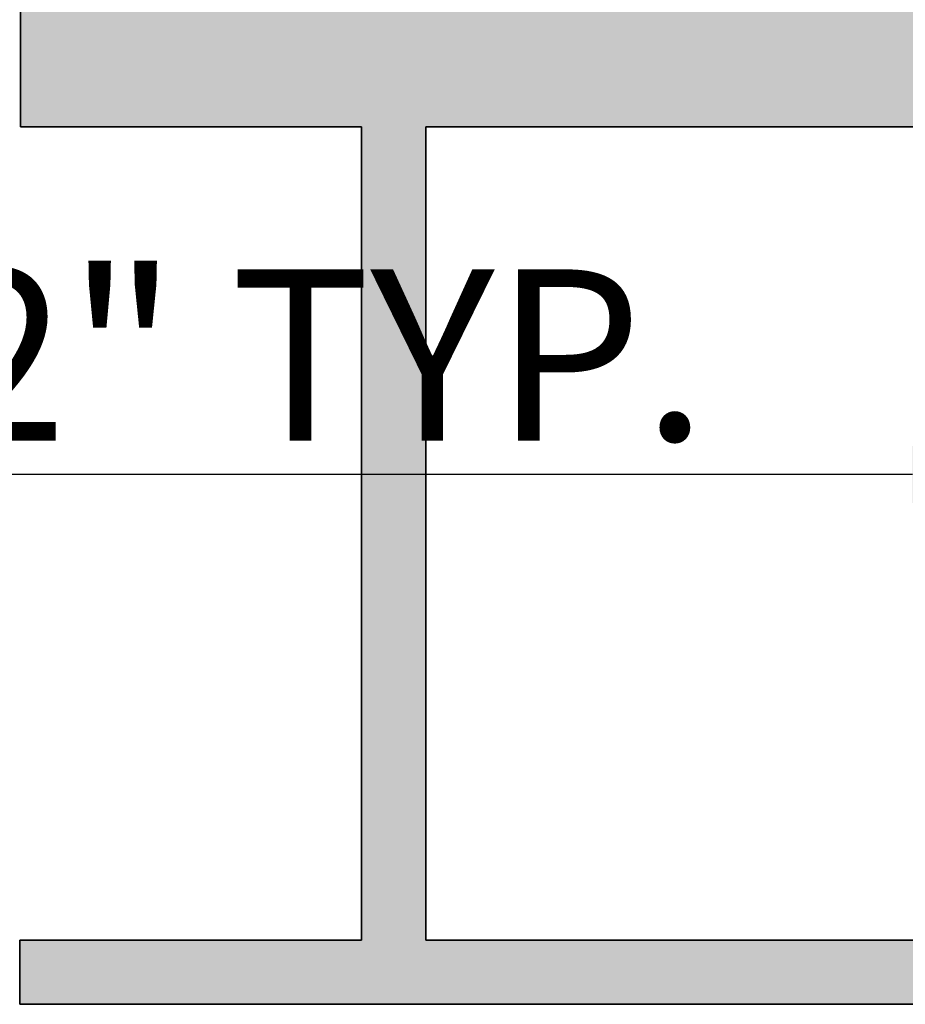
# Model space of a CAD drawing. Units: inches. Extents: x 2083 to 3317, y 1141 to 2115.
# Tile 246 of 256: x 2944 to 3006, y 1416 to 1485. Entities that reach past the tile are written whole.
import ezdxf

# ---------------------------------------------------------------- set-up
doc = ezdxf.new("R2010")
doc.units = ezdxf.units.IN
doc.layers.add('A-ANNO-DIMS', color=2, linetype='Continuous', lineweight=18)
doc.layers.add('A-WALL', color=7, linetype='Continuous', lineweight=35)
doc.layers.add('A-WALL-PATT', color=251, linetype='Continuous', lineweight=13, true_color=0x636466)
doc.styles.get("Standard").update_dxf_attribs({"font": 'arial.ttf'})
doc.dimstyles.new('ISO-25', dxfattribs={"dimtxt": 12, "dimasz": 12, "dimexe": 1.25, "dimexo": 0.625, "dimtad": 1, "dimlunit": 3, "dimtxsty": 'Standard', "dimcen": 2.5, "dimadec": 0, "dimazin": 0, "dimtfac": 1, "dimtmove": 0, "dimatfit": 3, "dimfxl": 1, "dimarcsym": 0})

# ---------------------------------------------------------------- blocks, each defined once
blk = doc.blocks.new('*D18')
at = {"layer": 'A-ANNO-DIMS', "color": 0, "lineweight": -2, "transparency": 16777216}
for p, q in [((3018.476, 1456.156), (3018.476, 1452.142)), ((3041.068, 1456.156), (3041.068, 1452.142)), ((3006.476, 1453.392), (2828.361, 1453.392)), ((3041.068, 1453.392), (3018.476, 1453.392)), ((3053.068, 1453.392), (3065.068, 1453.392))]:
    blk.add_line(p, q, dxfattribs=at)
at = {"layer": 'A-ANNO-DIMS', "color": 0, "transparency": 16777216}
for points in [[(3006.476, 1455.392), (3006.476, 1451.392), (3018.476, 1453.392)], [(3053.068, 1455.392), (3053.068, 1451.392), (3041.068, 1453.392)]]:
    blk.add_solid(points, dxfattribs=at)
at = {"layer": 'Defpoints', "color": 0, "transparency": 16777216}
for p in [(3018.476, 1456.781), (3041.068, 1456.781), (3018.476, 1453.392)]:
    blk.add_point(p, dxfattribs=at)
at = {"layer": 'A-ANNO-DIMS', "color": 0, "transparency": 16777216, "insert": (2911.418, 1460.222), "char_height": 12, "attachment_point": 5}
blk.add_mtext('BASIN 1\'-10 1/2" TYP.', dxfattribs=at)
blk = doc.blocks.new('*D73')
at = {"layer": 'A-ANNO-DIMS', "color": 0, "lineweight": -2, "transparency": 16777216}
for p, q in [((2895.865, 1420.763), (2930.553, 1387.52)), ((2980.105, 1340.032), (2939.217, 1379.217))]:
    blk.add_line(p, q, dxfattribs=at)
at = {"layer": 'A-ANNO-DIMS', "color": 0, "transparency": 16777216}
blk.add_solid([(2940.601, 1380.661), (2937.833, 1377.773), (2930.553, 1387.52)], dxfattribs=at)
at = {"layer": 'Defpoints', "color": 0, "transparency": 16777216}
for p in [(2895.865, 1420.763), (2930.553, 1387.52)]:
    blk.add_point(p, dxfattribs=at)
at = {"layer": 'A-ANNO-DIMS', "color": 0, "transparency": 16777216, "insert": (2968.665, 1360.348), "char_height": 12, "attachment_point": 5, "rotation": 316.21871}
blk.add_mtext('R4\'-0"', dxfattribs=at)

msp = doc.modelspace()

# ---------------------------------------------------------------- hatches: boundary and pattern name
at = {"layer": 'A-WALL-PATT'}
h = msp.add_hatch(color=256, dxfattribs=at)
h.dxf.hatch_style = 1
h.paths.add_polyline_path([(3126.96, 2020.761), (2748.96, 2020.761), (2604.96, 2020.761), (2226.96, 2020.761), (2226.96, 1702.761), (2466.96, 1702.761), (2466.96, 1582.761), (2418.96, 1582.761), (2418.96, 1477.761), (2226.96, 1477.761), (2226.96, 1263.261), (2544.96, 1263.261), (2544.96, 1411.761), (2604.96, 1411.761), (2685.96, 1411.761), (2685.96, 1420.761), (2604.96, 1420.761), (2604.96, 1573.761), (2604.96, 1702.761), (2604.96, 2011.761), (2748.96, 2011.761), (2748.96, 1702.761), (2862.96, 1702.761), (2862.96, 1621.761), (2871.96, 1621.761), (2871.96, 1702.761), (2883.96, 1702.761), (2883.96, 1706.939, -0.026459), (2883.96, 1711.761), (2757.96, 1711.761), (2757.96, 1807.761), (2787.96, 1807.761), (2787.96, 1812.261), (2757.96, 1812.261), (2757.96, 2011.761), (2877.96, 2011.761), (2877.96, 1812.261), (2847.96, 1812.261), (2847.96, 1807.761), (2889.836, 1807.761), (2889.836, 1812.261), (2882.46, 1812.261), (2882.46, 2011.761), (3117.96, 2011.761), (3117.96, 1812.261), (2937.836, 1812.261), (2937.836, 1807.761), (2995.71, 1807.761), (2995.71, 1796.118), (3000.21, 1796.118), (3000.21, 1807.761), (3117.96, 1807.761), (3117.96, 1711.761), (3000.21, 1711.761), (3000.21, 1760.118), (2998.573, 1760.118, -0.020711), (2995.71, 1760.118), (2995.71, 1711.761), (2931.96, 1711.761), (2931.96, 1702.761), (3126.96, 1702.761)])
h.paths.add_polyline_path([(2471.46, 2011.761), (2471.46, 1810.011), (2462.717, 1810.011), (2462.717, 1805.511), (2505.96, 1805.511), (2505.96, 1810.011), (2475.96, 1810.011), (2475.96, 2011.761), (2595.96, 2011.761), (2595.96, 1810.011), (2565.96, 1810.011), (2565.96, 1805.511), (2595.96, 1805.511), (2595.96, 1711.761), (2235.96, 1711.761), (2235.96, 1805.511), (2353.71, 1805.511), (2353.71, 1796.054), (2358.21, 1796.054), (2358.21, 1805.511), (2414.717, 1805.511), (2414.717, 1810.011), (2235.96, 1810.011), (2235.96, 2011.761)], flags=16)
h.paths.add_polyline_path([(2270.205, 1994.61), (2270.205, 1970.61), (2246.205, 1970.61), (2246.205, 1994.61)], flags=0)
edge = h.paths.add_edge_path(flags=0)
edge.add_ellipse((2332.027, 1899.798), major_axis=(-3.043, 3.043), ratio=0.168252, start_angle=-161.33217, end_angle=-156.30711, ccw=False)
edge.add_ellipse((2333.082, 1898.744), major_axis=(-1.055, 1.055), ratio=0.453532, start_angle=-123.37102, end_angle=-94.15911)
edge = h.paths.add_edge_path(flags=0)
edge.add_ellipse((2332.027, 1968.876), major_axis=(3.043, 3.043), ratio=0.168252, start_angle=18.66783, end_angle=23.69289)
edge.add_spline(control_points=[(2332.926, 1970.691), (2332.227, 1970.336), (2330.894, 1969.659), (2328.413, 1970.932), (2327.204, 1967.749), (2324.71, 1969.956), (2322.533, 1967.012), (2320.013, 1971.296), (2317.68, 1968.158), (2316.041, 1967.102), (2315.427, 1966.81)], knot_values=[0, 0, 0, 0, 2.267059, 4.324559, 6.685584, 8.878641, 11.121502, 14.300359, 17.755284, 19.732645, 19.732645, 19.732645, 19.732645], degree=3, periodic=0)
edge.add_ellipse((2332.027, 1968.876), major_axis=(3.043, 3.043), ratio=0.168252, start_angle=18.66783, end_angle=23.69289, ccw=False)
edge.add_ellipse((2333.082, 1969.931), major_axis=(1.055, 1.055), ratio=0.453532, start_angle=56.62898, end_angle=85.84089, ccw=False)
edge = h.paths.add_edge_path(flags=0)
edge.add_spline(control_points=[(2296.428, 1967.988), (2293.628, 1965.336), (2287.704, 1959.727), (2299.744, 1949.996), (2294.533, 1935.669), (2290.573, 1920.604), (2293.394, 1909.974), (2296.185, 1904.967)], knot_values=[0.099185, 0.099185, 0.099185, 0.099185, 0.345301, 0.619822, 0.982653, 1.386093, 1.810555, 1.810555, 1.810555, 1.810555], degree=3, periodic=0)
edge.add_spline(control_points=[(2296.185, 1904.967), (2297.384, 1902.619), (2298.001, 1901.949), (2298.553, 1901.468)], knot_values=[0.006246, 0.006246, 0.006246, 0.006246, 0.055476, 0.055476, 0.055476, 0.055476], degree=3, periodic=0)
edge.add_spline(control_points=[(2298.553, 1901.468), (2297.259, 1900.923), (2295.225, 1900.232), (2293.06, 1900.614), (2292.101, 1900.788), (2292.09, 1900.791)], knot_values=[0.312835, 0.312835, 0.312835, 0.312835, 0.40178, 0.474987, 0.475903, 0.475903, 0.475903, 0.475903], degree=3, periodic=0)
edge.add_arc((2292.794, 1904.664), 3.937, 215.4209, 259.69818, ccw=False)
edge.add_spline(control_points=[(2289.585, 1902.382), (2289.477, 1902.535), (2289.368, 1902.688), (2289.261, 1902.841)], knot_values=[0.102872, 0.102872, 0.102872, 0.102872, 0.116896, 0.116896, 0.116896, 0.116896], degree=3, periodic=0)
edge.add_spline(control_points=[(2289.261, 1902.841), (2288.687, 1902.55), (2287.64, 1902.02), (2285.881, 1901.874), (2283.853, 1901.504), (2281.72, 1899.711), (2278.467, 1899.493), (2276.157, 1901.883), (2272.259, 1899.804), (2267.778, 1901.843), (2262.244, 1900.184), (2257.415, 1901.782), (2254.318, 1900.726), (2253.178, 1900.337)], knot_values=[0, 0, 0, 0, 1.907977, 3.477176, 5.261074, 7.972851, 11.680248, 13.717921, 16.939592, 22.789562, 27.502503, 33.595215, 37.145618, 37.145618, 37.145618, 37.145618], degree=3, periodic=0)
edge.add_line((2253.178, 1900.337), (2250.244, 1902.841))
edge.add_line((2250.244, 1902.841), (2250.244, 1965.833))
edge.add_line((2250.244, 1965.833), (2253.178, 1968.337))
edge.add_spline(control_points=[(2253.178, 1968.337), (2254.318, 1967.948), (2257.415, 1966.892), (2262.244, 1968.49), (2267.778, 1966.831), (2271.527, 1968.537), (2273.876, 1967.828), (2274.207, 1967.728)], knot_values=[0, 0, 0, 0, 0.09018, 0.244935, 0.364644, 0.513233, 0.537855, 0.537855, 0.537855, 0.537855], degree=3, periodic=0)
edge.add_arc((2274.353, 1963.793), 3.937, 72.05113, 92.12795, ccw=False)
edge.add_arc((2281.297, 1985.23), 18.596, 252.05113, 288.56572)
edge.add_arc((2292.317, 1956.029), 12.646, 71.02679, 113.77822, ccw=False)
edge = h.paths.add_edge_path(flags=0)
edge.add_spline(control_points=[(2274.899, 1951.856), (2275.066, 1951.617), (2275.233, 1951.377), (2275.398, 1951.136)], knot_values=[1.409916, 1.409916, 1.409916, 1.409916, 1.43159, 1.43159, 1.43159, 1.43159], degree=3, periodic=0)
edge.add_spline(control_points=[(2275.398, 1951.136), (2275.792, 1950.562), (2276.179, 1949.984), (2276.546, 1949.397)], knot_values=[1.358238, 1.358238, 1.358238, 1.358238, 1.409916, 1.409916, 1.409916, 1.409916], degree=3, periodic=0)
edge.add_line((2276.546, 1949.397), (2277.437, 1947.862))
edge.add_spline(control_points=[(2277.437, 1947.862), (2276.304, 1945.673), (2274.64, 1942.427), (2274.632, 1938.094), (2272.799, 1930.852), (2274.356, 1943.897), (2275.948, 1947.923), (2276.546, 1949.397)], knot_values=[0.005632, 0.005632, 0.005632, 0.005632, 0.186014, 0.266002, 0.357087, 0.59639, 0.739732, 0.739732, 0.739732, 0.739732], degree=3, periodic=0)
edge.add_spline(control_points=[(2276.546, 1949.397), (2276.179, 1949.984), (2275.792, 1950.562), (2275.398, 1951.136)], knot_values=[1.358238, 1.358238, 1.358238, 1.358238, 1.409916, 1.409916, 1.409916, 1.409916], degree=3, periodic=0)
edge.add_spline(control_points=[(2275.398, 1951.136), (2274.943, 1950.08), (2274.208, 1948.025), (2273.935, 1944.851), (2272.469, 1937.627), (2273.466, 1945.696), (2274.701, 1951.059), (2274.899, 1951.856)], knot_values=[0.104364, 0.104364, 0.104364, 0.104364, 0.189636, 0.269624, 0.36071, 0.600013, 0.644622, 0.644622, 0.644622, 0.644622], degree=3, periodic=0)
h.paths.add_polyline_path([(2269.168, 1963.128, -0.357527), (2268.171, 1960.976, -0.092561), (2268.171, 1939.436, -0.357527), (2269.168, 1937.285, -0.357527), (2267.016, 1938.282, -0.164785), (2254.686, 1938.282, -0.357527), (2252.534, 1937.285, -0.357527), (2253.531, 1939.436, -0.092561), (2253.531, 1960.976, -0.357527), (2252.534, 1963.128, -0.357527), (2254.686, 1962.131, -0.164785), (2267.016, 1962.131, -0.357527)], flags=0)
h.paths.add_polyline_path([(2248.874, 1967.802), (2248.874, 1957.028), (2249.458, 1957.028), (2249.458, 1911.647), (2248.874, 1911.647), (2248.874, 1900.873), (2246.512, 1900.873, 0.197327), (2244.15, 1902.457), (2244.15, 1966.218, 0.197327), (2246.512, 1967.802)], flags=0)
h.paths.add_polyline_path([(2269.168, 1931.389, -0.357527), (2268.171, 1929.238, -0.092561), (2268.171, 1907.698, -0.357527), (2269.168, 1905.547, -0.357527), (2267.016, 1906.544, -0.164785), (2254.686, 1906.544, -0.357527), (2252.534, 1905.547, -0.357527), (2253.531, 1907.698, -0.092561), (2253.531, 1929.238, -0.357527), (2252.534, 1931.389, -0.357527), (2254.686, 1930.392, -0.164785), (2267.016, 1930.392, -0.357527)], flags=0)
edge = h.paths.add_edge_path(flags=0)
edge.add_spline(control_points=[(2276.197, 1906.724), (2276.168, 1909.029), (2276.114, 1913.372), (2270.598, 1924.925), (2273.905, 1919.013), (2275.922, 1916.262), (2275.475, 1912.402), (2277.258, 1910.381), (2276.696, 1908.225), (2276.646, 1906.813), (2276.618, 1906.008)], knot_values=[0, 0, 0, 0, 8.61026, 16.221274, 18.843057, 23.804898, 27.440828, 29.356102, 31.203478, 33.650687, 33.650687, 33.650687, 33.650687], degree=3, periodic=0)
edge.add_spline(control_points=[(2276.618, 1906.008), (2276.623, 1905.624), (2276.498, 1904.629), (2275.442, 1903.855), (2274.937, 1903.08), (2274.859, 1902.841)], knot_values=[0.156488, 0.156488, 0.156488, 0.156488, 0.184398, 0.231376, 0.250598, 0.250598, 0.250598, 0.250598], degree=3, periodic=0)
edge.add_line((2274.859, 1902.841), (2276.506, 1902.841))
edge.add_spline(control_points=[(2276.506, 1902.841), (2276.788, 1903.085), (2277.665, 1904.125), (2278.25, 1904.341), (2277.654, 1908.527), (2278.156, 1906.228), (2278.1, 1905.286), (2278.847, 1904.069), (2277.857, 1903.415), (2277.874, 1902.991), (2277.904, 1902.841)], knot_values=[0.059574, 0.059574, 0.059574, 0.059574, 0.080753, 0.103741, 0.16972, 0.176036, 0.207137, 0.240474, 0.262341, 0.27366, 0.27366, 0.27366, 0.27366], degree=3, periodic=0)
edge.add_line((2277.904, 1902.841), (2280.03, 1902.841))
edge.add_spline(control_points=[(2280.03, 1902.841), (2279.888, 1903.088), (2279.499, 1903.982), (2280.152, 1905.939), (2278.104, 1909.658), (2279.762, 1907.185), (2280.328, 1904.875), (2280.485, 1903.49), (2281.463, 1903.249), (2281.758, 1902.936), (2281.834, 1902.841)], knot_values=[0.013856, 0.013856, 0.013856, 0.013856, 0.034874, 0.088867, 0.107879, 0.126738, 0.158714, 0.193757, 0.217487, 0.226722, 0.226722, 0.226722, 0.226722], degree=3, periodic=0)
edge.add_spline(control_points=[(2281.834, 1902.841), (2281.788, 1902.827), (2281.647, 1902.783), (2281.396, 1902.859), (2281.088, 1902.985), (2280.721, 1903.061), (2280.333, 1903.026), (2280.125, 1902.899), (2280.03, 1902.841)], knot_values=[0, 0, 0, 0, 0.14413, 0.435517, 0.749276, 1.153046, 1.548371, 1.878348, 1.878348, 1.878348, 1.878348], degree=3, periodic=0)
edge.add_line((2280.03, 1902.841), (2277.904, 1902.841))
edge.add_spline(control_points=[(2277.904, 1902.841), (2277.893, 1902.796), (2277.865, 1902.68), (2277.607, 1902.687), (2277.274, 1902.801), (2276.838, 1902.62), (2276.584, 1902.789), (2276.506, 1902.841)], knot_values=[0, 0, 0, 0, 0.127189, 0.326199, 0.628009, 1.24357, 1.515331, 1.515331, 1.515331, 1.515331], degree=3, periodic=0)
edge.add_line((2276.506, 1902.841), (2274.859, 1902.841))
edge.add_spline(control_points=[(2274.859, 1902.841), (2274.814, 1902.899), (2274.725, 1903.013), (2274.493, 1903.119), (2274.244, 1902.961), (2273.937, 1903.185), (2273.614, 1902.983), (2273.408, 1902.883), (2273.322, 1902.841)], knot_values=[0, 0, 0, 0, 0.21843, 0.436957, 0.687977, 0.990379, 1.398396, 1.69185, 1.69185, 1.69185, 1.69185], degree=3, periodic=0)
edge.add_spline(control_points=[(2273.322, 1902.841), (2273.617, 1903.446), (2274.274, 1904.538), (2276.027, 1904.574), (2276.207, 1906.584), (2276.197, 1906.724)], knot_values=[0.012227, 0.012227, 0.012227, 0.012227, 0.059472, 0.106218, 0.134458, 0.134458, 0.134458, 0.134458], degree=3, periodic=0)
h.paths.add_polyline_path([(2270.776, 1897.79), (2270.776, 1873.79), (2246.776, 1873.79), (2246.776, 1897.79)], flags=0)
h.paths.add_polyline_path([(2353.71, 1760.005), (2353.71, 1760.054), (2358.21, 1760.054, -0.033729)], flags=0)
h.paths.add_polyline_path([(2321.819, 1737.529), (2341.995, 1737.529, -0.414214), (2343.203, 1736.321), (2343.203, 1721.021, -0.414214), (2341.995, 1719.813), (2321.819, 1719.813, -0.414214), (2320.611, 1721.021), (2320.611, 1736.321, -0.414214)], flags=0)
h.paths.add_polyline_path([(2324.235, 1736.321), (2339.579, 1736.321, -0.414214), (2341.995, 1733.905), (2341.995, 1725.45, -0.414214), (2339.579, 1723.034), (2333.681, 1723.034), (2333.845, 1722.045, -0.870646), (2335.425, 1721.826, -0.767327), (2333.923, 1721.423), (2331.291, 1721.423, -0.767327), (2329.788, 1721.826, -0.870646), (2331.368, 1722.045), (2331.533, 1723.034), (2324.235, 1723.034, -0.414214), (2321.819, 1725.45), (2321.819, 1733.905, -0.414214)], flags=0)
h.paths.add_polyline_path([(2570.484, 1928.615), (2589.684, 1928.615), (2590.169, 1928.615), (2590.169, 1904.993), (2570.484, 1904.993)], flags=0)
h.paths.add_polyline_path([(2574.447, 1927.264, -1), (2572.829, 1927.264, -1)], flags=0)
h.paths.add_polyline_path([(2573.09, 1926.941), (2573.925, 1927.776), (2574.148, 1927.553), (2573.313, 1926.718)], flags=0)
h.paths.add_polyline_path([(2578.779, 1919.73, -1), (2571.592, 1919.73, -1)], flags=0)
h.paths.add_polyline_path([(2578.385, 1919.73, -1), (2571.985, 1919.73, -1)], flags=0)
h.paths.add_polyline_path([(2331.596, 1729.476, -1), (2333.618, 1729.476, -1)], flags=0)
h.paths.add_polyline_path([(2578.034, 1927.264, -1), (2576.416, 1927.264, -1)], flags=0)
h.paths.add_polyline_path([(2576.689, 1927.531), (2576.912, 1927.754), (2577.747, 1926.919), (2577.524, 1926.696)], flags=0)
h.paths.add_polyline_path([(2578.139, 1909.86, -1), (2572.232, 1909.86, -1)], flags=0)
h.paths.add_polyline_path([(2577.745, 1909.86, -1), (2572.625, 1909.86, -1)], flags=0)
h.paths.add_polyline_path([(2583.798, 1927.264, -1), (2582.179, 1927.264, -1)], flags=0)
h.paths.add_polyline_path([(2582.719, 1927.754), (2583.554, 1926.919), (2583.331, 1926.696), (2582.496, 1927.531)], flags=0)
h.paths.add_polyline_path([(2582.496, 1927.531), (2582.719, 1927.754), (2583.554, 1926.919), (2583.331, 1926.696)], flags=0)
h.paths.add_polyline_path([(2587.739, 1920.53, -1), (2581.832, 1920.53, -1)], flags=0)
h.paths.add_polyline_path([(2587.345, 1920.53, -1), (2582.225, 1920.53, -1)], flags=0)
h.paths.add_polyline_path([(2587.385, 1927.264, -1), (2585.766, 1927.264, -1)], flags=0)
h.paths.add_polyline_path([(2586.082, 1926.98), (2586.917, 1927.815), (2587.14, 1927.593), (2586.305, 1926.758)], flags=0)
h.paths.add_polyline_path([(2588.379, 1910.66, -1), (2581.192, 1910.66, -1)], flags=0)
h.paths.add_polyline_path([(2587.985, 1910.66, -1), (2581.585, 1910.66, -1)], flags=0)
h.paths.add_polyline_path([(2417.168, 1729.478), (2437.344, 1729.478, -0.414214), (2438.552, 1728.27), (2438.552, 1712.969, -0.414214), (2437.344, 1711.761), (2417.168, 1711.761, -0.414214), (2415.96, 1712.969), (2415.96, 1728.27, -0.414214)], flags=0)
h.paths.add_polyline_path([(2419.584, 1728.27), (2434.928, 1728.27, -0.414214), (2437.344, 1725.854), (2437.344, 1717.398, -0.414214), (2434.928, 1714.983), (2429.029, 1714.983), (2429.194, 1713.994, -0.870646), (2430.774, 1713.775, -0.767327), (2429.271, 1713.372), (2426.64, 1713.372, -0.767327), (2425.137, 1713.775, -0.870646), (2426.717, 1713.994), (2426.882, 1714.983), (2419.584, 1714.983, -0.414214), (2417.168, 1717.398), (2417.168, 1725.854, -0.414214)], flags=0)
h.paths.add_polyline_path([(2419.584, 1728.27), (2434.928, 1728.27, -0.414214), (2437.344, 1725.854), (2437.344, 1717.398, -0.414214), (2434.928, 1714.983), (2429.029, 1714.983), (2428.358, 1719.009), (2427.553, 1719.009), (2426.882, 1714.983), (2419.584, 1714.983, -0.414214), (2417.168, 1717.398), (2417.168, 1725.854, -0.414214)], flags=0)
h.paths.add_polyline_path([(2426.944, 1721.425, -1), (2428.967, 1721.425, -1)], flags=0)
h.paths.add_polyline_path([(2475.96, 1702.761), (2595.96, 1702.761), (2595.96, 1582.761), (2475.96, 1582.761)], flags=16)
h.paths.add_polyline_path([(2427.96, 1573.761), (2595.96, 1573.761), (2595.96, 1468.761), (2595.96, 1420.761), (2384.46, 1420.761), (2384.46, 1468.761), (2427.96, 1468.761)], flags=16)
h.paths.add_polyline_path([(2379.96, 1468.761), (2379.96, 1420.761), (2235.96, 1420.761), (2235.96, 1468.761)], flags=16)
h.paths.add_polyline_path([(2317.816, 1466.696), (2337.992, 1466.696, -0.414214), (2339.2, 1465.488), (2339.2, 1450.187, -0.414214), (2337.992, 1448.979), (2317.816, 1448.979, -0.414214), (2316.608, 1450.187), (2316.608, 1465.488, -0.414214)], flags=0)
h.paths.add_polyline_path([(2320.232, 1465.488), (2335.576, 1465.488, -0.414214), (2337.992, 1463.072), (2337.992, 1454.616, -0.414214), (2335.576, 1452.2), (2329.677, 1452.2), (2329.842, 1451.212, -0.870646), (2331.422, 1450.992, -0.767327), (2329.92, 1450.59), (2327.288, 1450.59, -0.767327), (2325.785, 1450.992, -0.870646), (2327.365, 1451.212), (2327.53, 1452.2), (2320.232, 1452.2, -0.414214), (2317.816, 1454.616), (2317.816, 1463.072, -0.414214)], flags=0)
h.paths.add_polyline_path([(2320.232, 1465.488), (2335.576, 1465.488, -0.414214), (2337.992, 1463.072), (2337.992, 1454.616, -0.414214), (2335.576, 1452.2), (2329.677, 1452.2), (2329.006, 1456.227), (2328.201, 1456.227), (2327.53, 1452.2), (2320.232, 1452.2, -0.414214), (2317.816, 1454.616), (2317.816, 1463.072, -0.414214)], flags=0)
h.paths.add_polyline_path([(2327.593, 1458.643, -1), (2329.615, 1458.643, -1)], flags=0)
h.paths.add_polyline_path([(2244.412, 1433.34), (2241.921, 1433.34, -0.414214), (2240.018, 1435.244), (2240.018, 1440.953, -0.414211), (2241.921, 1442.856), (2244.412, 1442.856, -1.976472)], flags=0)
h.paths.add_polyline_path([(2245.357, 1434.398, -0.414214), (2245.357, 1441.799, -2.144098)], flags=0)
h.paths.add_polyline_path([(2535.96, 1416.261), (2535.96, 1272.261), (2235.96, 1272.261), (2235.96, 1416.261)], flags=16)
h.paths.add_polyline_path([(2260.12, 1384.293), (2260.12, 1362.039), (2237.865, 1362.039), (2237.865, 1384.293)], flags=0)
edge = h.paths.add_edge_path(flags=0)
edge.add_line((2318.252, 1362.093), (2318.146, 1362.001))
edge.add_ellipse((2317.445, 1360.431), major_axis=(2.822, 2.822), ratio=0.168252, start_angle=18.66783, end_angle=20.94813, ccw=False)
edge.add_ellipse((2318.423, 1361.409), major_axis=(0.978, 0.978), ratio=0.453532, start_angle=56.62898, end_angle=70.2262, ccw=False)
edge = h.paths.add_edge_path(flags=0)
edge.add_line((2319.107, 1295.571), (2319.015, 1295.677))
edge.add_ellipse((2317.445, 1296.378), major_axis=(-2.822, 2.822), ratio=0.168252, start_angle=-161.33217, end_angle=-159.05187, ccw=False)
edge.add_ellipse((2318.423, 1295.4), major_axis=(-0.978, 0.978), ratio=0.453532, start_angle=-123.37102, end_angle=-109.7738)
edge = h.paths.add_edge_path(flags=0)
edge.add_spline(control_points=[(2284.21, 1301.17), (2284.581, 1300.445), (2284.891, 1299.892), (2285.16, 1299.461)], knot_values=[0.039066, 0.039066, 0.039066, 0.039066, 0.055476, 0.055476, 0.055476, 0.055476], degree=3, periodic=0)
edge.add_line((2285.16, 1299.461), (2284.21, 1301.17))
edge = h.paths.add_edge_path(flags=0)
edge.add_line((2280.412, 1297.298), (2283.37, 1297.036))
edge.add_line((2283.37, 1297.036), (2286.406, 1297.926))
edge.add_spline(control_points=[(2286.406, 1297.926), (2285.305, 1297.463), (2284.345, 1297.129), (2283.37, 1297.036)], knot_values=[0.394369, 0.394369, 0.394369, 0.394369, 0.475903, 0.475903, 0.475903, 0.475903], degree=3, periodic=0)
edge.add_spline(control_points=[(2283.37, 1297.036), (2283.281, 1297.028), (2282.316, 1296.957), (2281.313, 1297.134), (2280.423, 1297.296), (2280.412, 1297.298)], knot_values=[0.312835, 0.312835, 0.312835, 0.312835, 0.320246, 0.393453, 0.394369, 0.394369, 0.394369, 0.394369], degree=3, periodic=0)
edge = h.paths.add_edge_path(flags=0)
edge.add_line((2284.436, 1359.607), (2280.446, 1355.328))
edge.add_line((2280.446, 1355.328), (2279.58, 1351.018))
edge.add_line((2279.58, 1351.018), (2282.413, 1346.58))
edge.add_spline(control_points=[(2282.413, 1346.58), (2283.153, 1345.589), (2284.253, 1344.029), (2284.801, 1342.387), (2284.935, 1341.806)], knot_values=[1.240098, 1.240098, 1.240098, 1.240098, 1.332892, 1.382712, 1.382712, 1.382712, 1.382712], degree=3, periodic=0)
edge.add_spline(control_points=[(2284.935, 1341.806), (2285.319, 1340.141), (2285.233, 1338.409), (2284.91, 1336.654)], knot_values=[1.097484, 1.097484, 1.097484, 1.097484, 1.240098, 1.240098, 1.240098, 1.240098], degree=3, periodic=0)
edge.add_spline(control_points=[(2284.91, 1336.654), (2284.587, 1334.899), (2284.027, 1333.12), (2283.463, 1331.361)], knot_values=[0.95487, 0.95487, 0.95487, 0.95487, 1.097484, 1.097484, 1.097484, 1.097484], degree=3, periodic=0)
edge.add_line((2283.463, 1331.361), (2281.89, 1326.153))
edge.add_line((2281.89, 1326.153), (2280.756, 1321.056))
edge.add_line((2280.756, 1321.056), (2280.299, 1316.002))
edge.add_line((2280.299, 1316.002), (2280.716, 1310.95))
edge.add_line((2280.716, 1310.95), (2282.028, 1305.972))
edge.add_line((2282.028, 1305.972), (2284.21, 1301.17))
edge.add_spline(control_points=[(2284.21, 1301.17), (2283.341, 1302.73), (2282.612, 1304.336), (2282.028, 1305.972)], knot_values=[0.099185, 0.099185, 0.099185, 0.099185, 0.241799, 0.241799, 0.241799, 0.241799], degree=3, periodic=0)
edge.add_spline(control_points=[(2282.028, 1305.972), (2281.444, 1307.608), (2281.005, 1309.273), (2280.716, 1310.95)], knot_values=[0.241799, 0.241799, 0.241799, 0.241799, 0.384413, 0.384413, 0.384413, 0.384413], degree=3, periodic=0)
edge.add_spline(control_points=[(2280.716, 1310.95), (2280.433, 1312.588), (2280.289, 1314.277), (2280.299, 1315.962), (2280.299, 1316.002)], knot_values=[0.384413, 0.384413, 0.384413, 0.384413, 0.523647, 0.527028, 0.527028, 0.527028, 0.527028], degree=3, periodic=0)
edge.add_spline(control_points=[(2280.299, 1316.002), (2280.312, 1317.687), (2280.478, 1319.368), (2280.756, 1321.056)], knot_values=[0.527028, 0.527028, 0.527028, 0.527028, 0.669642, 0.669642, 0.669642, 0.669642], degree=3, periodic=0)
edge.add_spline(control_points=[(2280.756, 1321.056), (2281.035, 1322.744), (2281.426, 1324.44), (2281.89, 1326.153)], knot_values=[0.669642, 0.669642, 0.669642, 0.669642, 0.812256, 0.812256, 0.812256, 0.812256], degree=3, periodic=0)
edge.add_spline(control_points=[(2281.89, 1326.153), (2282.264, 1327.533), (2282.788, 1329.262), (2283.353, 1331.018), (2283.463, 1331.361)], knot_values=[0.812256, 0.812256, 0.812256, 0.812256, 0.927087, 0.95487, 0.95487, 0.95487, 0.95487], degree=3, periodic=0)
edge.add_line((2283.463, 1331.361), (2284.91, 1336.654))
edge.add_line((2284.91, 1336.654), (2284.935, 1341.806))
edge.add_line((2284.935, 1341.806), (2282.413, 1346.58))
edge.add_spline(control_points=[(2282.413, 1346.58), (2281.275, 1348.104), (2280.078, 1349.57), (2279.58, 1351.018)], knot_values=[1.382712, 1.382712, 1.382712, 1.382712, 1.525326, 1.525326, 1.525326, 1.525326], degree=3, periodic=0)
edge.add_spline(control_points=[(2279.58, 1351.018), (2279.443, 1351.415), (2279.136, 1352.857), (2279.735, 1354.29), (2280.446, 1355.328)], knot_values=[1.525326, 1.525326, 1.525326, 1.525326, 1.564439, 1.667941, 1.667941, 1.667941, 1.667941], degree=3, periodic=0)
edge.add_spline(control_points=[(2280.446, 1355.328), (2281.426, 1356.758), (2282.931, 1358.183), (2284.436, 1359.607)], knot_values=[1.667941, 1.667941, 1.667941, 1.667941, 1.810555, 1.810555, 1.810555, 1.810555], degree=3, periodic=0)
edge.add_arc((2280.623, 1348.518), 11.726, 71.02679, 113.77822)
edge.add_arc((2270.405, 1375.595), 17.244, 252.05113, 288.56572, ccw=False)
edge.add_arc((2263.966, 1355.718), 3.651, 72.05113, 92.12795)
edge.add_arc((2263.966, 1355.718), 3.651, 92.12795, 177.98513)
edge.add_spline(control_points=[(2260.318, 1355.846), (2260.26, 1354.221), (2260.551, 1350.187), (2262.999, 1346.766), (2264.473, 1344.649)], knot_values=[1.43159, 1.43159, 1.43159, 1.43159, 1.564144, 1.770695, 1.770695, 1.770695, 1.770695], degree=3, periodic=0)
edge.add_line((2264.473, 1344.649), (2264.936, 1343.983))
edge.add_spline(control_points=[(2263.801, 1340.248), (2263.843, 1340.514), (2264.067, 1341.756), (2264.513, 1343.002), (2264.935, 1343.981)], knot_values=[0.53657, 0.53657, 0.53657, 0.53657, 0.559349, 0.644622, 0.644622, 0.644622, 0.644622], degree=3, periodic=0)
edge.add_spline(control_points=[(2264.935, 1343.981), (2265.118, 1343.715), (2265.299, 1343.448), (2265.477, 1343.179)], knot_values=[1.384077, 1.384077, 1.384077, 1.384077, 1.409916, 1.409916, 1.409916, 1.409916], degree=3, periodic=0)
edge.add_spline(control_points=[(2265.477, 1343.179), (2265.655, 1342.911), (2265.829, 1342.641), (2265.999, 1342.369)], knot_values=[1.358238, 1.358238, 1.358238, 1.358238, 1.384077, 1.384077, 1.384077, 1.384077], degree=3, periodic=0)
edge.add_line((2265.999, 1342.369), (2266.826, 1340.946))
edge.add_spline(control_points=[(2266.826, 1340.946), (2268.894, 1337.09), (2271.398, 1325.843), (2270.516, 1310.569), (2275.919, 1301.861), (2277.79, 1299.199)], knot_values=[0.116896, 0.116896, 0.116896, 0.116896, 0.472987, 1.050969, 1.313793, 1.313793, 1.313793, 1.313793], degree=3, periodic=0)
edge.add_spline(control_points=[(2277.79, 1299.199), (2277.839, 1299.128), (2277.889, 1299.057), (2277.94, 1298.987)], knot_values=[0.109884, 0.109884, 0.109884, 0.109884, 0.116896, 0.116896, 0.116896, 0.116896], degree=3, periodic=0)
edge.add_line((2277.94, 1298.987), (2277.789, 1299.199))
edge.add_spline(control_points=[(2277.789, 1299.199), (2277.257, 1298.929), (2276.286, 1298.438), (2275.039, 1298.334), (2274.383, 1298.239), (2274.215, 1298.209)], knot_values=[33.12187, 33.12187, 33.12187, 33.12187, 35.029056, 36.598255, 37.144827, 37.144827, 37.144827, 37.144827], degree=3, periodic=0)
edge.add_line((2274.215, 1298.209), (2273.073, 1297.893))
edge.add_spline(control_points=[(2273.073, 1297.893), (2272.323, 1297.58), (2271.039, 1296.511), (2269.248, 1296.226), (2268.423, 1296.375)], knot_values=[26.532584, 26.532584, 26.532584, 26.532584, 29.198919, 31.839101, 31.839101, 31.839101, 31.839101], degree=3, periodic=0)
edge.add_line((2268.423, 1296.375), (2263.879, 1297.458))
edge.add_spline(control_points=[(2263.879, 1297.458), (2263.556, 1297.359), (2261.86, 1296.839), (2260.239, 1297.282), (2258.933, 1297.516)], knot_values=[15.919551, 15.919551, 15.919551, 15.919551, 16.939592, 21.226067, 21.226067, 21.226067, 21.226067], degree=3, periodic=0)
edge.add_line((2258.933, 1297.516), (2254.055, 1297.329))
edge.add_spline(control_points=[(2254.055, 1297.329), (2253.756, 1297.296), (2252.114, 1297.165), (2250.462, 1297.544), (2249.13, 1297.668)], knot_values=[5.306517, 5.306517, 5.306517, 5.306517, 6.276435, 10.613034, 10.613034, 10.613034, 10.613034], degree=3, periodic=0)
edge.add_line((2249.13, 1297.668), (2244.332, 1296.878))
edge.add_line((2244.332, 1296.878), (2241.611, 1299.199))
edge.add_line((2241.611, 1299.199), (2241.611, 1357.609))
edge.add_line((2241.611, 1357.609), (2244.332, 1359.931))
edge.add_line((2244.332, 1359.931), (2252.729, 1359.543))
edge.add_spline(control_points=[(2252.729, 1359.543), (2252.871, 1359.546), (2253.306, 1359.548), (2253.74, 1359.514), (2254.032, 1359.482)], knot_values=[0.233291, 0.233291, 0.233291, 0.233291, 0.244935, 0.268927, 0.268927, 0.268927, 0.268927], degree=3, periodic=0)
edge.add_line((2254.032, 1359.482), (2259.587, 1359.416))
edge.add_spline(control_points=[(2259.587, 1359.416), (2260.677, 1359.629), (2262.073, 1359.897), (2263.524, 1359.459), (2263.83, 1359.366)], knot_values=[0.422516, 0.422516, 0.422516, 0.422516, 0.513233, 0.537855, 0.537855, 0.537855, 0.537855], degree=3, periodic=0)
edge.add_arc((2263.966, 1355.718), 3.651, 72.05113, 92.12795, ccw=False)
edge.add_arc((2270.405, 1375.595), 17.244, 252.05113, 288.56572)
edge.add_arc((2280.623, 1348.518), 11.726, 71.02679, 113.77822, ccw=False)
h.paths.add_polyline_path([(2240.341, 1359.435), (2240.341, 1349.444), (2240.882, 1349.444), (2240.882, 1307.365), (2240.341, 1307.365), (2240.341, 1297.374), (2238.15, 1297.374, 0.197327), (2235.96, 1298.843), (2235.96, 1357.966, 0.197327), (2238.15, 1359.435)], flags=0)
h.paths.add_polyline_path([(2259.158, 1355.101, -0.357527), (2258.233, 1353.106, -0.092561), (2258.233, 1333.133, -0.357527), (2259.158, 1331.138, -0.357527), (2257.163, 1332.062, -0.164785), (2245.729, 1332.062, -0.357527), (2243.735, 1331.138, -0.357527), (2244.659, 1333.133, -0.092561), (2244.659, 1353.106, -0.357527), (2243.735, 1355.101, -0.357527), (2245.729, 1354.176, -0.164785), (2257.163, 1354.176, -0.357527)], flags=0)
edge = h.paths.add_edge_path(flags=0)
edge.add_line((2265.999, 1342.369), (2266.826, 1340.946))
edge.add_line((2266.826, 1340.946), (2265.308, 1337.814))
edge.add_line((2265.308, 1337.814), (2264.358, 1334.653))
edge.add_line((2264.358, 1334.653), (2264.262, 1333.8))
edge.add_spline(control_points=[(2264.262, 1333.8), (2264.208, 1333.187), (2264.162, 1332.366), (2264.007, 1331.414), (2263.969, 1331.202)], knot_values=[0.464444, 0.464444, 0.464444, 0.464444, 0.516691, 0.531608, 0.531608, 0.531608, 0.531608], degree=3, periodic=0)
edge.add_spline(control_points=[(2263.969, 1331.202), (2263.775, 1330.119), (2263.424, 1328.791), (2263.257, 1328.531), (2263.234, 1328.515)], knot_values=[0.372682, 0.372682, 0.372682, 0.372682, 0.44885, 0.464444, 0.464444, 0.464444, 0.464444], degree=3, periodic=0)
edge.add_spline(control_points=[(2263.234, 1328.515), (2263.096, 1328.42), (2263.131, 1329.301), (2263.275, 1330.616)], knot_values=[0.280919, 0.280919, 0.280919, 0.280919, 0.372682, 0.372682, 0.372682, 0.372682], degree=3, periodic=0)
edge.add_spline(control_points=[(2263.275, 1330.616), (2263.419, 1331.93), (2263.672, 1333.677), (2263.97, 1335.315)], knot_values=[0.189157, 0.189157, 0.189157, 0.189157, 0.280919, 0.280919, 0.280919, 0.280919], degree=3, periodic=0)
edge.add_spline(control_points=[(2263.97, 1335.315), (2264.1, 1336.032), (2264.419, 1337.622), (2264.755, 1338.864), (2264.947, 1339.491)], knot_values=[0.097394, 0.097394, 0.097394, 0.097394, 0.137578, 0.189157, 0.189157, 0.189157, 0.189157], degree=3, periodic=0)
edge.add_spline(control_points=[(2264.947, 1339.491), (2265.29, 1340.606), (2265.644, 1341.494), (2265.999, 1342.369)], knot_values=[0.005632, 0.005632, 0.005632, 0.005632, 0.097394, 0.097394, 0.097394, 0.097394], degree=3, periodic=0)
h.paths.add_polyline_path([(2259.158, 1325.671, -0.357527), (2258.233, 1323.676, -0.092561), (2258.233, 1303.703, -0.357527), (2259.158, 1301.708, -0.357527), (2257.163, 1302.633, -0.164785), (2245.729, 1302.633, -0.357527), (2243.735, 1301.708, -0.357527), (2244.659, 1303.703, -0.092561), (2244.659, 1323.676, -0.357527), (2243.735, 1325.671, -0.357527), (2245.729, 1324.747, -0.164785), (2257.163, 1324.747, -0.357527)], flags=0)
edge = h.paths.add_edge_path(flags=0)
edge.add_spline(control_points=[(2261.709, 1317.311), (2261.679, 1317.418), (2261.762, 1317.389), (2262.491, 1316.09), (2262.962, 1315.301)], knot_values=[14.955861, 14.955861, 14.955861, 14.955861, 16.221274, 18.694826, 18.694826, 18.694826, 18.694826], degree=3, periodic=0)
edge.add_spline(control_points=[(2262.962, 1315.301), (2262.99, 1315.254), (2263.702, 1314.067), (2264.349, 1313.127), (2264.73, 1312.164)], knot_values=[18.694826, 18.694826, 18.694826, 18.694826, 18.843057, 22.433791, 22.433791, 22.433791, 22.433791], degree=3, periodic=0)
edge.add_spline(control_points=[(2264.73, 1312.164), (2264.876, 1311.796), (2265.177, 1310.77), (2265.143, 1309.559), (2265.248, 1308.824)], knot_values=[22.433791, 22.433791, 22.433791, 22.433791, 23.804898, 26.172756, 26.172756, 26.172756, 26.172756], degree=3, periodic=0)
edge.add_line((2265.248, 1308.824), (2265.851, 1307.172))
edge.add_spline(control_points=[(2265.851, 1307.172), (2266.065, 1306.822), (2266.384, 1306.332), (2266.424, 1305.781), (2266.42, 1305.611)], knot_values=[28.062562, 28.062562, 28.062562, 28.062562, 29.356102, 29.911721, 29.911721, 29.911721, 29.911721], degree=3, periodic=0)
edge.add_spline(control_points=[(2266.42, 1305.611), (2266.416, 1305.433), (2266.394, 1305.25), (2266.365, 1305.066)], knot_values=[29.911721, 29.911721, 29.911721, 29.911721, 30.497837, 30.497837, 30.497837, 30.497837], degree=3, periodic=0)
edge.add_line((2266.365, 1305.066), (2266.066, 1302.136))
edge.add_spline(control_points=[(2266.066, 1302.136), (2266.071, 1301.78), (2265.998, 1301.2), (2265.663, 1300.759), (2265.509, 1300.586)], knot_values=[0.156488, 0.156488, 0.156488, 0.156488, 0.184398, 0.203543, 0.203543, 0.203543, 0.203543], degree=3, periodic=0)
edge.add_line((2265.509, 1300.586), (2264.435, 1299.199))
edge.add_line((2264.435, 1299.199), (2265.962, 1299.199))
edge.add_line((2265.962, 1299.199), (2267.336, 1301.175))
edge.add_line((2267.336, 1301.175), (2267.312, 1301.986))
edge.add_spline(control_points=[(2267.312, 1301.986), (2267.261, 1302.862), (2267.16, 1303.737), (2267.271, 1303.326)], knot_values=[0.126229, 0.126229, 0.126229, 0.126229, 0.166617, 0.166617, 0.166617, 0.166617], degree=3, periodic=0)
edge.add_spline(control_points=[(2267.271, 1303.326), (2267.28, 1303.294), (2267.31, 1303.175), (2267.373, 1302.884), (2267.406, 1302.683), (2267.418, 1302.601)], knot_values=[0.166617, 0.166617, 0.166617, 0.166617, 0.16972, 0.176036, 0.180765, 0.180765, 0.180765, 0.180765], degree=3, periodic=0)
edge.add_spline(control_points=[(2267.744, 1300.988), (2267.688, 1301.151), (2267.481, 1301.657), (2267.484, 1302.145), (2267.418, 1302.601)], knot_values=[0.180765, 0.180765, 0.180765, 0.180765, 0.193767, 0.220139, 0.220139, 0.220139, 0.220139], degree=3, periodic=0)
edge.add_line((2267.418, 1302.601), (2267.744, 1300.988))
edge.add_spline(control_points=[(2267.744, 1300.988), (2267.832, 1300.732), (2267.932, 1300.31), (2267.555, 1299.975), (2267.429, 1299.829)], knot_values=[0.220139, 0.220139, 0.220139, 0.220139, 0.240474, 0.25489, 0.25489, 0.25489, 0.25489], degree=3, periodic=0)
edge.add_line((2267.429, 1299.829), (2267.258, 1299.199))
edge.add_line((2267.258, 1299.199), (2269.23, 1299.199))
edge.add_spline(control_points=[(2269.23, 1299.199), (2269.099, 1299.429), (2268.843, 1300.016), (2269.012, 1300.916), (2268.947, 1301.661)], knot_values=[0.013856, 0.013856, 0.013856, 0.013856, 0.034874, 0.067073, 0.067073, 0.067073, 0.067073], degree=3, periodic=0)
edge.add_line((2268.947, 1301.661), (2268.432, 1303.603))
edge.add_spline(control_points=[(2268.432, 1303.603), (2268.176, 1304.192), (2267.596, 1305.251), (2268.041, 1304.623), (2268.251, 1304.282)], knot_values=[0.090155, 0.090155, 0.090155, 0.090155, 0.107879, 0.120289, 0.120289, 0.120289, 0.120289], degree=3, periodic=0)
edge.add_spline(control_points=[(2268.251, 1304.282), (2268.361, 1304.105), (2269.058, 1302.918), (2269.383, 1301.59), (2269.521, 1300.776), (2269.575, 1300.556)], knot_values=[0.120289, 0.120289, 0.120289, 0.120289, 0.126738, 0.158714, 0.173506, 0.173506, 0.173506, 0.173506], degree=3, periodic=0)
edge.add_line((2269.575, 1300.556), (2270.686, 1299.421))
edge.add_spline(control_points=[(2270.686, 1299.421), (2270.767, 1299.357), (2270.838, 1299.281), (2270.903, 1299.199)], knot_values=[0.21816, 0.21816, 0.21816, 0.21816, 0.226722, 0.226722, 0.226722, 0.226722], degree=3, periodic=0)
edge.add_line((2270.937, 1299.193), (2270.903, 1299.199))
edge.add_spline(control_points=[(2270.903, 1299.199), (2270.86, 1299.186), (2270.73, 1299.146), (2270.496, 1299.216), (2270.272, 1299.308), (2270.121, 1299.348), (2270.063, 1299.36)], knot_values=[0.939174, 0.939174, 0.939174, 0.939174, 1.083304, 1.374691, 1.68845, 1.878348, 1.878348, 1.878348, 1.878348], degree=3, periodic=0)
edge.add_line((2270.063, 1299.36), (2269.23, 1299.199))
edge.add_line((2269.23, 1299.199), (2267.258, 1299.199))
edge.add_spline(control_points=[(2267.258, 1299.199), (2267.248, 1299.157), (2267.223, 1299.05), (2266.984, 1299.057), (2266.809, 1299.116), (2266.677, 1299.109), (2266.637, 1299.105)], knot_values=[0.757665, 0.757665, 0.757665, 0.757665, 0.884854, 1.083864, 1.385675, 1.515331, 1.515331, 1.515331, 1.515331], degree=3, periodic=0)
edge.add_spline(control_points=[(2266.637, 1299.105), (2266.485, 1299.089), (2266.236, 1299.017), (2266.035, 1299.151), (2265.962, 1299.199)], knot_values=[0, 0, 0, 0, 0.485905, 0.757665, 0.757665, 0.757665, 0.757665], degree=3, periodic=0)
edge.add_line((2265.962, 1299.199), (2264.435, 1299.199))
edge.add_line((2264.435, 1299.199), (2263.858, 1299.367))
edge.add_spline(control_points=[(2263.858, 1299.367), (2263.819, 1299.371), (2263.78, 1299.386), (2263.74, 1299.402)], knot_values=[0.845925, 0.845925, 0.845925, 0.845925, 0.978627, 0.978627, 0.978627, 0.978627], degree=3, periodic=0)
edge.add_line((2263.722, 1299.396), (2263.01, 1299.199))
edge.add_spline(control_points=[(2263.01, 1299.199), (2263.246, 1299.683), (2263.506, 1300.128), (2263.873, 1300.408)], knot_values=[0.012227, 0.012227, 0.012227, 0.012227, 0.052971, 0.052971, 0.052971, 0.052971], degree=3, periodic=0)
edge.add_spline(control_points=[(2263.873, 1300.408), (2263.932, 1300.453), (2264.084, 1300.553), (2264.255, 1300.624), (2264.36, 1300.665)], knot_values=[0.052971, 0.052971, 0.052971, 0.052971, 0.059472, 0.069086, 0.069086, 0.069086, 0.069086], degree=3, periodic=0)
edge.add_line((2264.36, 1300.665), (2265.142, 1301.078))
edge.add_line((2265.142, 1301.078), (2265.676, 1302.8))
edge.add_line((2265.676, 1302.8), (2265.541, 1305.704))
edge.add_line((2265.541, 1305.704), (2264.803, 1309.328))
edge.add_line((2264.803, 1309.328), (2263.041, 1314.092))
edge.add_spline(control_points=[(2263.041, 1314.092), (2262.384, 1315.671), (2261.796, 1316.998), (2261.709, 1317.311)], knot_values=[11.216896, 11.216896, 11.216896, 11.216896, 14.955861, 14.955861, 14.955861, 14.955861], degree=3, periodic=0)
h.paths.add_polyline_path([(2871.96, 1416.261), (2895.91, 1416.261), (2895.91, 1420.761), (2871.96, 1420.761), (2871.96, 1501.761), (2862.96, 1501.761), (2862.96, 1420.761), (2805.96, 1420.761), (2805.96, 1411.761), (2862.96, 1411.761), (2862.96, 1263.261), (3126.96, 1263.261), (3126.96, 1411.761), (3126.96, 1486.761), (2943.96, 1486.761), (2943.96, 1477.761), (2967.86, 1477.761), (2967.86, 1420.761), (2943.91, 1420.761), (2943.91, 1416.261), (3117.96, 1416.261), (3117.96, 1420.761), (2972.36, 1420.761), (2972.36, 1477.761), (3117.96, 1477.761), (3117.96, 1420.761), (3117.96, 1272.261), (2871.96, 1272.261)], flags=0)
h.paths.add_polyline_path([(2457.126, 1485.943), (2527.603, 1485.943), (2527.603, 1537.636), (2457.126, 1537.636)], flags=8)
h.paths.add_polyline_path([(2481.005, 1609.982), (2590.766, 1609.982), (2590.766, 1682.003), (2481.005, 1682.003)], flags=8)
h.paths.add_polyline_path([(2483.085, 1729.127), (2553.562, 1729.127), (2553.562, 1780.82), (2483.085, 1780.82)], flags=8)
h = msp.add_hatch(color=256, dxfattribs=at)
h.dxf.hatch_style = 1
h.paths.add_polyline_path([(3126.96, 1486.761), (2943.96, 1486.761), (2943.96, 1477.761), (2967.86, 1477.761), (2967.86, 1420.761), (2943.91, 1420.761), (2943.91, 1416.261), (3117.96, 1416.261), (3117.96, 1420.761), (2972.36, 1420.761), (2972.36, 1477.761), (3117.96, 1477.761), (3117.96, 1420.761), (3117.96, 1272.261), (2871.96, 1272.261), (2871.96, 1416.261), (2895.91, 1416.261), (2895.91, 1420.761), (2871.96, 1420.761), (2871.96, 1501.761), (2862.96, 1501.761), (2862.96, 1420.761), (2805.96, 1420.761), (2805.96, 1411.761), (2862.96, 1411.761), (2862.96, 1263.261), (3126.96, 1263.261), (3126.96, 1411.761)])

# ---------------------------------------------------------------- linework, layer by layer
at = {"layer": 'A-WALL'}
for p, q in [((2943.96, 1702.761), (2943.96, 1477.761)), ((2943.96, 1477.761), (2967.86, 1477.761)), ((2967.86, 1477.761), (2967.86, 1420.761)), ((2972.36, 1477.761), (2972.36, 1420.761)), ((2972.36, 1477.761), (3117.96, 1477.761)), ((2943.91, 1420.761), (2943.91, 1416.261)), ((2943.91, 1420.761), (2967.86, 1420.761)), ((2972.36, 1420.761), (3117.96, 1420.761)), ((2943.91, 1416.261), (3117.96, 1416.261))]:
    msp.add_line(p, q, dxfattribs=at)

# ---------------------------------------------------------------- dimensions: what is measured, and where the dimension line sits
at = {"layer": 'A-ANNO-DIMS'}
dim = msp.add_linear_dim(base=(3018.476, 1453.392), p1=(3041.068, 1456.781), p2=(3018.476, 1456.781), angle=180, text='BASIN <> TYP.', dimstyle='ISO-25', override={"dimdec": 1, "dimlfac": 1, "dimrnd": 0, "dimzin": 1, "dimdsep": 46, "dimlunit": 4, "dimfrac": 2}, dxfattribs=at)
dim.commit()
dim.dimension.update_dxf_attribs({"geometry": '*D18', "text_midpoint": (2911.418, 1460.222)})
dim = msp.add_radius_dim(center=(2895.865, 1420.763), mpoint=(2930.553, 1387.52), dimstyle='ISO-25', override={"dimdec": 1, "dimlfac": 1, "dimrnd": 0, "dimzin": 1, "dimdsep": 46, "dimlunit": 4, "dimfrac": 2}, dxfattribs=at)
dim.commit()
dim.dimension.update_dxf_attribs({"geometry": '*D73', "text_midpoint": (2968.665, 1360.348)})

doc.saveas('drawing.dxf')
